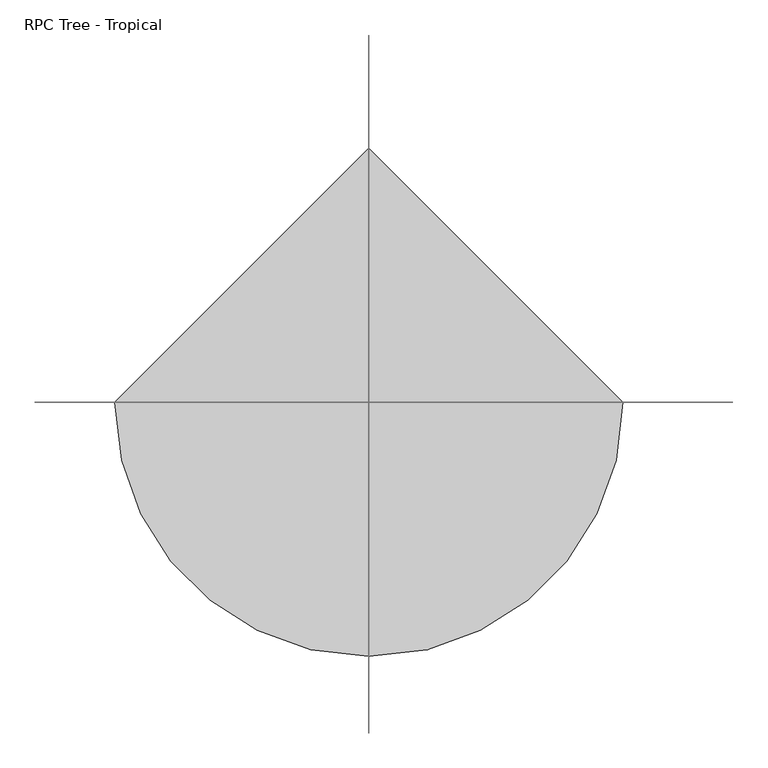
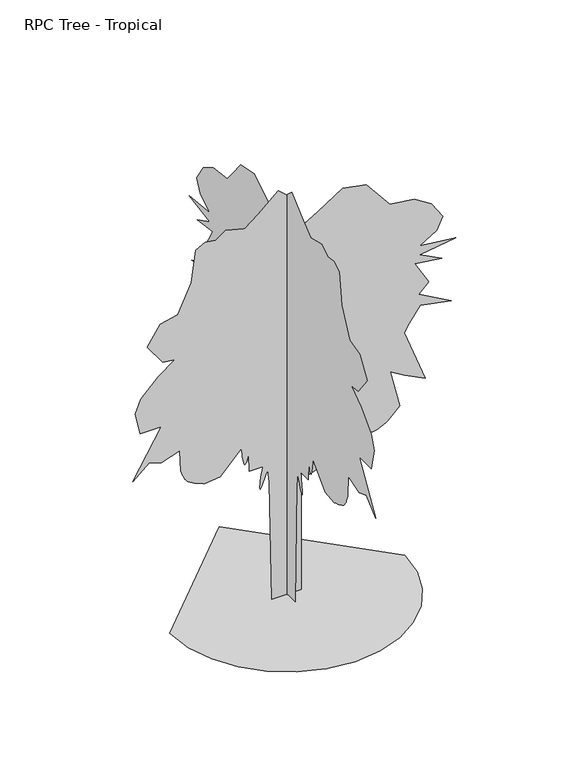
"""IFC4 building model written with IfcOpenShell, lengths in millimetres: geographic element geometry, RPC Tree - Tropical."""

from ifc_helpers import new_model, si_unit, origin, place, context, project, spatial, triangles, source, transform, mapped, element, save


def rpc_tree_tropical_d7a905c7(model_context):
    return source(origin(), model_context, "Body", "Tessellation", [
        triangles([(-0.2241189, -80.6803134, 0.0560704), (-0.2241181, -93.4507094, 708.3955685), (-0.2241176, -102.9729479, 784.5729681), (-0.2241171, -112.4304103, 759.6428038), (-0.2241163, -121.4992608, 736.1299221), (-0.2241158, -129.7908604, 715.4466642), (-0.2241156, -136.916343, 699.0127836), (-0.2241151, -142.4870876, 688.2406214), (-0.2241151, -146.1147278, 684.5474602), (-0.2241148, -147.4101338, 689.3505827), (-0.2241148, -146.9475984, 700.5392893), (-0.2241151, -145.6519381, 714.7252693), (-0.2241151, -143.662352, 731.4105881), (-0.2241153, -141.1175219, 750.0923693), (-0.2241156, -138.1563745, 770.2752216), (-0.2241156, -134.9173553, 791.458885), (-0.2241158, -131.5396545, 813.1404104), (-0.2241113, -207.7180624, 813.1404104), (-0.224111, -210.8920511, 914.7103008), (-0.2241108, -214.9636775, 900.580204), (-0.2241105, -218.9799477, 887.367057), (-0.2241105, -222.88496, 875.9827955), (-0.2241103, -226.6235945, 867.3493109), (-0.22411, -230.1402221, 862.3810095), (-0.2241097, -233.3789961, 861.9923704), (-0.2241095, -236.2847599, 867.1003435), (-0.2241095, -238.9129061, 876.4653969), (-0.2241092, -241.3744383, 887.9944897), (-0.2241092, -243.6972616, 901.3295042), (-0.224109, -245.9088635, 916.1097794), (-0.224109, -248.0373855, 931.9696398), (-0.2241087, -250.1102786, 948.5533659), (-0.2241087, -252.1552483, 965.4977531), (-0.2241016, -372.7715778, 838.5329012), (-0.2240963, -461.6464946, 829.010372), (-0.224095, -479.2563572, 835.8125004), (-0.224094, -496.4217339, 842.6147015), (-0.2240932, -512.6981023, 849.4168299), (-0.2240922, -527.64352, 856.2164148), (-0.2240914, -540.8134646, 863.0185432), (-0.2240907, -551.7608706, 869.8206717), (-0.2240902, -560.0413244, 876.6228727), (-0.2240899, -566.4726179, 884.1641275), (-0.2240897, -572.238436, 893.0389492), (-0.2240892, -577.4480018, 903.0236595), (-0.2240889, -582.2155887, 913.8974871), (-0.2240887, -586.6479126, 925.4367537), (-0.2240884, -590.8567037, 937.4204699), (-0.2240881, -594.9562717, 949.6252481), (-0.2240879, -601.3062839, 1073.4150759), (-0.2240815, -706.0511621, 1038.5001286), (-0.2240775, -775.8810568, 1063.8925467), (-0.2240719, -867.928418, 981.3677147), (-0.2240815, -706.0511621, 1254.3398609), (-0.2240744, -826.6659657, 1254.3398609), (-0.2240727, -855.233408, 1381.3021694), (-0.2240747, -823.4909414, 1460.6545933), (-0.2240805, -725.0961479, 1562.224411), (-0.2240861, -629.8712191, 1632.0567764), (-0.2240821, -699.7011137, 1641.5768349), (-0.224077, -785.4035133, 1759.0190849), (-0.2240813, -712.3985945, 1873.2865288), (-0.2240871, -614.0012575, 1895.5039227), (-0.2240917, -537.8238579, 2060.5586735), (-0.2240932, -512.4314034, 2247.8284927), (-0.2240963, -458.4714704, 2276.3959351), (-0.2240998, -398.1640686, 2266.8734058), (-0.2241034, -341.0291113, 2308.1358582), (-0.2241097, -233.1107712, 2279.5708866), (-0.2241143, -156.9326267, 2339.8783974), (-0.2241212, -42.6652782, 2438.2757343), (-0.2241265, 46.2093524, 2358.9233105), (-0.2241265, 46.2093524, 2263.6984543), (-0.2241298, 103.3427746, 2190.6960789), (-0.2241346, 182.6954255, 2235.1334827), (-0.224143, 322.3549604, 2327.1809166), (-0.2241509, 455.6672811, 2301.7884258), (-0.2241557, 538.1921494, 2200.2186081), (-0.2241588, 588.979638, 2136.7361458), (-0.2241672, 728.6394636, 2117.6910873), (-0.224173, 827.0368006, 2057.3837219), (-0.2241768, 890.5167194, 1958.986385), (-0.2241748, 855.6017721, 1889.1564903), (-0.2241689, 760.3793867, 1828.8489796), (-0.2241811, 963.5216383, 1806.6315857), (-0.2241689, 760.3793867, 1774.8890465), (-0.2241763, 884.1692144, 1711.4067295), (-0.2241674, 731.8118717, 1730.4516426), (-0.224172, 811.1642956, 1593.9668049), (-0.2241687, 754.0318817, 1540.0068718), (-0.2241796, 938.1291475, 1435.2621025), (-0.2241692, 763.5544109, 1470.1769772), (-0.2241654, 700.0719486, 1384.477121), (-0.2241636, 671.5045063, 1336.8647655), (-0.224171, 792.1193098, 1022.630167), (-0.2241639, 674.6795305, 1079.7650517), (-0.224159, 592.1520824, 1130.5500332), (-0.2241621, 646.1120155, 908.3627958), (-0.2241583, 579.4571451, 841.7079254), (-0.2241575, 566.5462689, 834.2758209), (-0.2241567, 553.721761, 827.1511105), (-0.224156, 541.0623593, 820.6359558), (-0.2241552, 528.6518887, 815.0378237), (-0.2241544, 516.5766809, 810.6613466), (-0.2241537, 504.9155105, 807.8089771), (-0.2241532, 493.7572526, 806.7929054), (-0.2241524, 482.6879065, 807.6260668), (-0.2241519, 471.2883479, 809.9577559), (-0.2241511, 459.6093733, 813.5392233), (-0.2241504, 447.7094456, 818.1188129), (-0.2241496, 435.6418682, 823.4503189), (-0.2241489, 423.4625244, 829.2796143), (-0.2241481, 411.2298409, 835.357877), (-0.2241481, 407.7779803, 839.4116993), (-0.2241478, 404.0213056, 843.2979446), (-0.2241476, 399.6524952, 846.8514341), (-0.2241471, 394.3692784, 849.9070616), (-0.2241468, 387.8643339, 852.2946339), (-0.2241463, 379.8302676, 853.8491175), (-0.2241458, 369.9674249, 854.4028627), (-0.224145, 357.1403735, 855.883659), (-0.224144, 340.8157522, 860.0289728), (-0.2241428, 321.5777186, 866.3967527), (-0.2241415, 300.0079778, 874.5400057), (-0.2241402, 276.6881621, 884.0168255), (-0.2241387, 252.2014664, 894.3800737), (-0.2241372, 227.1326114, 905.1877716), (-0.2241349, 185.8694142, 857.577887), (-0.2241349, 185.8694142, 778.2254631), (-0.2241362, 208.0876256, 702.0480635), (-0.2241316, 131.9097354, 676.6556454), (-0.2241288, 87.4725496, 800.4429296), (-0.2241293, 88.096376, 0.0), (-666.8181644, -2.5e-06, 0.2128606), (-649.2007078, -152.6793797, 0.2128611), (-599.0329851, -292.8908795, 0.2128626), (-520.3257617, -416.61723, 0.2128649), (-417.1023385, -519.8431603, 0.2128679), (-293.3760243, -598.5478403, 0.2128717), (-153.1642702, -648.715563, 0.2128758), (-0.4850755, -666.3330196, 0.2128804), (152.1942349, -648.715563, 0.2128849), (292.4057347, -598.5478403, 0.212889), (416.1320852, -519.8406169, 0.2128928), (519.3580155, -416.61723, 0.2128959), (598.0626955, -292.8908795, 0.2128981), (648.2304182, -152.6791254, 0.2128997), (665.8478748, 5.82e-05, 0.2129002), (-0.4851924, 666.3330196, 0.2128804), (-89.341994, 0.0001455, 0.1894216), (-102.11239, 0.0001057, 708.5276825), (-111.6346285, 9.96e-05, 784.7075529), (-121.0920909, 0.0001025, 759.7773886), (-130.1609414, 0.0001023, 736.2619635), (-138.4522867, 0.0001051, 715.581249), (-145.5777693, 0.000105, 699.144825), (-151.1487682, 0.0001048, 688.3726627), (-154.7761631, 0.0001075, 684.682045), (-156.0718144, 0.0001043, 689.4852402), (-155.6090338, 0.0001041, 700.6714033), (-154.3136187, 0.0001037, 714.8573833), (-152.3240326, 0.0001034, 731.5426294), (-149.7792025, 0.0001031, 750.2269541), (-146.8178008, 9.98e-05, 770.4098791), (-143.5790359, 9.95e-05, 791.590999), (-140.2013351, 9.92e-05, 813.2725245), (-216.3794887, 9.82e-05, 813.2725245), (-219.5534773, 9.2e-05, 914.8448856), (-223.6253582, 9.2e-05, 900.7147888), (-227.6413739, 9.5e-05, 887.4991711), (-231.5466406, 9.5e-05, 876.1173803), (-235.2852751, 9.49e-05, 867.4838957), (-238.8016665, 9.47e-05, 862.5131235), (-242.0406767, 9.44e-05, 862.1244844), (-244.9461861, 9.4e-05, 867.2324575), (-247.5745867, 9.35e-05, 876.5974382), (-250.0361189, 9.29e-05, 888.1290745), (-252.358706, 9.23e-05, 901.464089), (-254.5697811, 9.17e-05, 916.2418934), (-256.6983031, 9.1e-05, 932.1042246), (-258.7709418, 9.04e-05, 948.6854073), (-260.8156571, 8.97e-05, 965.6297945), (-381.4330041, 9.73e-05, 838.667486), (-470.3079208, 9.84e-05, 829.1450294), (-487.9177835, 9.66e-05, 835.9446144), (-505.0831601, 9.78e-05, 842.7467428), (-521.3595285, 9.61e-05, 849.5488712), (-536.3049462, 9.46e-05, 856.3510723), (-549.4748909, 9.61e-05, 863.1532007), (-560.4222968, 9.49e-05, 869.9527857), (-568.7027507, 9.4e-05, 876.7549141), (-575.1340442, 9.32e-05, 884.2962416), (-580.8998623, 9.24e-05, 893.1709906), (-586.109428, 9.17e-05, 903.1557735), (-590.8770149, 9.38e-05, 914.0295284), (-595.3093389, 9.31e-05, 925.568795), (-599.5181299, 9.23e-05, 937.5525839), (-603.617698, 9.16e-05, 949.759833), (-609.9677101, 8.15e-05, 1073.5496607), (-714.7125521, 8.49e-05, 1038.6347134), (-784.5424467, 8.37e-05, 1064.0272041), (-876.5898079, 8.96e-05, 981.4997561), (-714.7125521, 7.26e-05, 1254.4719749), (-835.3274282, 7.35e-05, 1254.4719749), (-863.8948706, 6.42e-05, 1381.4367542), (-832.152404, 5.89e-05, 1460.7891781), (-733.7575378, 5.3e-05, 1562.3589958), (-638.532609, 5.06e-05, 1632.1888905), (-708.3625763, 4.99e-05, 1641.7114197), (-794.0649759, 4.17e-05, 1759.1538151), (-721.0600571, 3.61e-05, 1873.4184975), (-622.6626474, 3.25e-05, 1895.6385075), (-546.4852841, 2.27e-05, 2060.6907875), (-521.0928297, 1.36e-05, 2247.9630775), (-467.1328966, 1.17e-05, 2276.5305199), (-406.8254949, 1.15e-05, 2267.0079906), (-349.6905375, 9.6e-06, 2308.270443), (-241.7724518, 1.13e-05, 2279.7030006), (-165.5940529, 7.6e-06, 2340.0103661), (-51.3267045, 3e-07, 2438.4078484), (37.5476695, 7.7e-06, 2359.0554245), (37.5476695, 1.34e-05, 2263.8330391), (94.6810849, 1.78e-05, 2190.8281929), (174.0337449, 1.48e-05, 2235.2655968), (313.6935342, 7e-06, 2327.3155014), (447.0058548, 1.09e-05, 2301.9230106), (529.5307231, 1.55e-05, 2200.3505768), (580.3182117, 1.9e-05, 2136.8682598), (719.978001, 2.04e-05, 2117.8258175), (818.3728672, 2.51e-05, 2057.515836), (881.8552568, 3.08e-05, 1959.1209698), (846.9403095, 3.56e-05, 1889.2910751), (751.7179241, 3.77e-05, 1828.9837097), (954.8601757, 3.9e-05, 1806.7636997), (751.7179241, 4.22e-05, 1775.0237766), (875.5077518, 4.35e-05, 1711.5413143), (723.1504818, 4.39e-05, 1730.5862274), (802.502833, 5.21e-05, 1594.0989189), (745.3704918, 5.45e-05, 1540.1416019), (929.4676849, 6.24e-05, 1435.3942165), (754.8929483, 6.03e-05, 1470.3117073), (691.4105587, 6.3e-05, 1384.609235), (662.8430437, 6.77e-05, 1336.9993504), (783.4579199, 8.5e-05, 1022.7647518), (666.0180679, 8.15e-05, 1079.8971657), (583.4906562, 7.85e-05, 1130.6820745), (637.4506256, 9.28e-05, 908.4973806), (570.7957189, 9.76e-05, 841.8399668), (557.8848427, 9.67e-05, 834.4104784), (545.0603348, 9.87e-05, 827.2831518), (532.4009331, 9.77e-05, 820.7706133), (519.9904624, 9.97e-05, 815.169865), (507.9152547, 9.88e-05, 810.7934607), (496.2540842, 9.78e-05, 807.9435619), (485.0932829, 9.98e-05, 806.9250195), (474.0264802, 9.87e-05, 807.7581808), (462.6269217, 9.77e-05, 810.0898699), (450.947947, 9.94e-05, 813.6712646), (439.0480193, 9.82e-05, 818.2534704), (426.980442, 9.7e-05, 823.5823603), (414.8010982, 9.86e-05, 829.4117283), (402.5684146, 9.74e-05, 835.4924618), (399.1165541, 9.69e-05, 839.5463568), (395.3598793, 9.65e-05, 843.4325294), (390.9910689, 9.6e-05, 846.9860189), (385.7078522, 9.54e-05, 850.0391029), (379.2029077, 9.48e-05, 852.4267479), (371.1688414, 9.69e-05, 853.9812315), (361.3059986, 9.6e-05, 854.5374475), (348.4789473, 9.48e-05, 856.0183165), (332.154326, 9.62e-05, 860.1635576), (312.9162924, 9.43e-05, 866.5288668), (291.3465516, 9.5e-05, 874.6721197), (268.0267359, 9.56e-05, 884.1488668), (243.5397858, 9.31e-05, 894.5146585), (218.4709308, 9.34e-05, 905.3224291), (177.2077336, 9.7e-05, 857.7099283), (177.2077336, 9.94e-05, 778.3575771), (199.4261993, 0.0001036, 702.1801775), (123.2483092, 0.0001063, 676.7876867), (78.8108599, 9.87e-05, 800.5775145), (79.4346863, 0.0001459, 0.1333563)], [[85, 84, 86], [53, 52, 54], [91, 90, 92], [87, 86, 88], [95, 94, 96], [96, 94, 97], [9, 8, 10], [52, 51, 54], [51, 50, 54], [1, 133, 2], [133, 132, 2], [2, 132, 3], [131, 130, 132], [130, 129, 132], [129, 128, 132], [18, 17, 19], [71, 70, 72], [72, 70, 73], [10, 8, 11], [8, 7, 11], [11, 7, 12], [7, 6, 12], [12, 6, 13], [6, 5, 13], [13, 5, 14], [5, 4, 14], [14, 4, 15], [4, 3, 15], [15, 3, 16], [16, 3, 17], [55, 54, 56], [89, 88, 90], [56, 54, 57], [57, 54, 58], [61, 60, 62], [62, 60, 63], [60, 59, 63], [25, 24, 26], [24, 23, 26], [26, 23, 27], [23, 22, 27], [27, 22, 28], [22, 21, 28], [28, 21, 29], [21, 20, 29], [29, 20, 30], [20, 19, 30], [30, 19, 31], [82, 81, 83], [83, 81, 84], [81, 80, 84], [80, 79, 84], [70, 69, 73], [98, 97, 99], [31, 19, 32], [99, 97, 100], [58, 54, 59], [100, 97, 101], [101, 97, 102], [102, 97, 103], [103, 97, 104], [104, 97, 105], [105, 97, 106], [106, 97, 107], [107, 97, 108], [108, 97, 109], [109, 97, 110], [110, 97, 111], [111, 97, 112], [112, 97, 113], [113, 97, 114], [114, 97, 115], [115, 97, 116], [116, 97, 117], [117, 97, 118], [118, 97, 119], [119, 97, 120], [120, 97, 121], [121, 97, 122], [122, 97, 123], [123, 97, 124], [124, 97, 125], [125, 97, 126], [126, 97, 127], [65, 64, 66], [66, 64, 67], [68, 67, 69], [67, 64, 69], [3, 132, 17], [73, 69, 74], [69, 64, 74], [64, 63, 74], [63, 59, 74], [17, 132, 19], [132, 128, 19], [128, 127, 19], [92, 90, 93], [76, 75, 77], [77, 75, 78], [78, 75, 79], [79, 75, 84], [75, 74, 84], [74, 59, 84], [84, 59, 86], [86, 59, 88], [88, 59, 90], [90, 59, 93], [93, 59, 94], [94, 59, 97], [97, 59, 127], [127, 59, 19], [32, 19, 33], [19, 59, 33], [59, 54, 33], [54, 50, 33], [33, 50, 34], [50, 49, 34], [34, 49, 35], [35, 49, 36], [36, 49, 37], [49, 48, 37], [37, 48, 38], [48, 47, 38], [38, 47, 39], [47, 46, 39], [39, 46, 40], [46, 45, 40], [45, 44, 40], [40, 44, 41], [44, 43, 41], [41, 43, 42], [148, 149, 134], [147, 148, 134], [147, 134, 135], [146, 147, 135], [146, 135, 136], [146, 136, 137], [145, 146, 137], [144, 145, 137], [144, 137, 138], [144, 138, 139], [144, 139, 140], [144, 140, 141], [144, 141, 142], [144, 142, 143], [233, 234, 235], [201, 202, 203], [239, 240, 241], [235, 236, 237], [243, 244, 245], [243, 245, 246], [157, 158, 159], [200, 201, 203], [199, 200, 203], [282, 150, 151], [281, 282, 151], [281, 151, 152], [279, 280, 281], [278, 279, 281], [277, 278, 281], [166, 167, 168], [219, 220, 221], [219, 221, 222], [157, 159, 160], [156, 157, 160], [156, 160, 161], [155, 156, 161], [155, 161, 162], [154, 155, 162], [154, 162, 163], [153, 154, 163], [153, 163, 164], [152, 153, 164], [152, 164, 165], [152, 165, 166], [203, 204, 205], [237, 238, 239], [203, 205, 206], [203, 206, 207], [209, 210, 211], [209, 211, 212], [208, 209, 212], [173, 174, 175], [172, 173, 175], [172, 175, 176], [171, 172, 176], [171, 176, 177], [170, 171, 177], [170, 177, 178], [169, 170, 178], [169, 178, 179], [168, 169, 179], [168, 179, 180], [230, 231, 232], [230, 232, 233], [229, 230, 233], [228, 229, 233], [218, 219, 222], [246, 247, 248], [168, 180, 181], [246, 248, 249], [203, 207, 208], [246, 249, 250], [246, 250, 251], [246, 251, 252], [246, 252, 253], [246, 253, 254], [246, 254, 255], [246, 255, 256], [246, 256, 257], [246, 257, 258], [246, 258, 259], [246, 259, 260], [246, 260, 261], [246, 261, 262], [246, 262, 263], [246, 263, 264], [246, 264, 265], [246, 265, 266], [246, 266, 267], [246, 267, 268], [246, 268, 269], [246, 269, 270], [246, 270, 271], [246, 271, 272], [246, 272, 273], [246, 273, 274], [246, 274, 275], [246, 275, 276], [213, 214, 215], [213, 215, 216], [216, 217, 218], [213, 216, 218], [281, 152, 166], [218, 222, 223], [213, 218, 223], [212, 213, 223], [208, 212, 223], [281, 166, 168], [277, 281, 168], [276, 277, 168], [239, 241, 242], [224, 225, 226], [224, 226, 227], [224, 227, 228], [224, 228, 233], [223, 224, 233], [208, 223, 233], [208, 233, 235], [208, 235, 237], [208, 237, 239], [208, 239, 242], [208, 242, 243], [208, 243, 246], [208, 246, 276], [208, 276, 168], [168, 181, 182], [208, 168, 182], [203, 208, 182], [199, 203, 182], [199, 182, 183], [198, 199, 183], [198, 183, 184], [198, 184, 185], [198, 185, 186], [197, 198, 186], [197, 186, 187], [196, 197, 187], [196, 187, 188], [195, 196, 188], [195, 188, 189], [194, 195, 189], [193, 194, 189], [193, 189, 190], [192, 193, 190], [192, 190, 191]], closed=False),
    ])


if __name__ == "__main__":
    model = new_model("IFC4")
    model_context = context("Model", 3, world=origin())
    ifc_project = project(units=[si_unit("LENGTHUNIT", "METRE", prefix="MILLI")], contexts=[model_context])
    site = spatial("IfcSite", under=ifc_project)
    building = spatial("IfcBuilding", under=site)
    placement = place(None, origin())
    rpc_tree_tropical_shape = rpc_tree_tropical_d7a905c7(model_context)
    element("IfcGeographicElement", 1, ObjectType="RPC Tree - Tropical", at=placement, inside=building, context=model_context, shape_type="MappedRepresentation", body=[
        mapped(rpc_tree_tropical_shape, transform((0.0, 0.0, 0.0), x_axis=(1.0, 0.0, 0.0), y_axis=(0.0, 1.0, 0.0), z_axis=(0.0, 0.0, 1.0))),
    ])
    save(model, "model.ifc")

# Revit data of these elements
# Type "RPC Tree - Tropical"
#   built-in parameter 1005198 = "{2, 15},{39, RPC-16-G2MF-J1Q0-CAN1-N000-ST1L-LVER-AU},{1, 0},{1, 0},{2, 13},{1, 8},{5, Color},{1, 0},{1, 0},{3, 0.8},{3, 0.8},{3, 0.8},{1, 8},{7, BBoxMin},{1, 0},{1, 0},{1, 0},{1, 0},{1, 0},{1, 8},{7, BBoxMax},{1, 0},{1, 0},{1, 0},{1, 0},{1, 0},{2, 11},{9, RPCTypeId},{1, 0},{1, 0},{39, RPC-16-G2MF-J1Q0-CAN1-N000-ST1L-LVER-AU},{1, 6},{14, RPCPlantHeight},{1, 0},{1, 0},{1, 8},{2, 11},{7, keyword},{1, 0},{1, 0},{35, :RPCs:Trees [Tropical]:Geometry:RPC},{2, 11},{8, category},{1, 0},{1, 0},{16, Trees [Tropical]},{2, 11},{12, LocalizedUID},{1, 0},{1, 0},{13, Windmill Palm},{2, 14},{6, Height},{1, 0},{1, 0},{1, 8},{1, 2},{16, Cast Reflections},{1, 0},{1, 0},{1, 0},{1, 2},{12, Cast Shadows},{1, 0},{1, 0},{1, 1},{1, 2},{9, Lock View},{1, 0},{1, 0},{1, 0},{1, 4},{5, ViewC},{1, 0},{1, 0},{1, 0},{21, assetlibrary_base.fbx},{1, 5},"
#   built-in parameter 1005195 = "RPC-16-G2MF-J1Q0-CAN1-N000-ST1L-LVER-AU"
#   Assembly Code = "G2050500"
#   Height = 8' - 0"
#   Plan Symbol = element 387627
#   Default Elevation = 0
